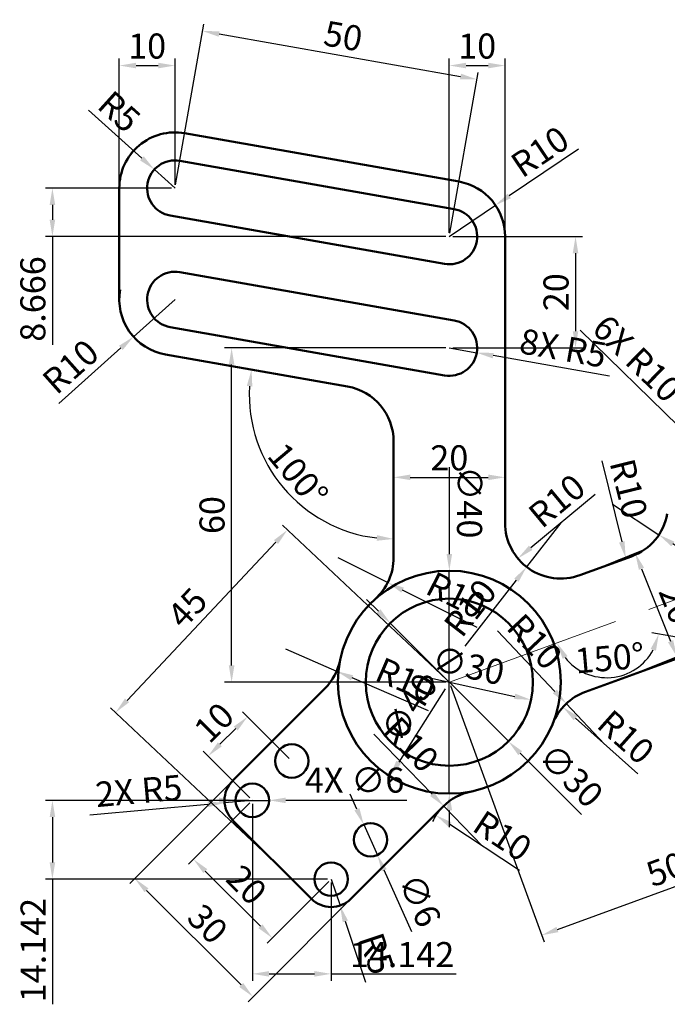
# Model space of a CAD drawing. Units: millimetres. Extents: x 54 to 254, y 16 to 193.
# Tile 1 of 2: x 54 to 170, y 16 to 193. Entities that reach past the tile are written whole.
import ezdxf

# ---------------------------------------------------------------- set-up
doc = ezdxf.new("R2010")
doc.units = ezdxf.units.MM
doc.linetypes.add('CENTER', pattern=[50.8, 31.75, -6.35, 6.35, -6.35])
for name, color, linetype, lineweight in [('M-CNTR', 1, 'CENTER', 18), ('M-DIMS', 2, 'Continuous', 25), ('M-OUTL', 7, 'Continuous', 50)]:
    doc.layers.add(name, color=color, linetype=linetype, lineweight=lineweight)
doc.styles.get("Standard").update_dxf_attribs({"font": 'arial.ttf'})
doc.dimstyles.new('ISO-25', dxfattribs={"dimtxt": 4.5, "dimasz": 3, "dimexe": 1.25, "dimexo": 0.625, "dimtad": 1, "dimdec": 0, "dimtxsty": 'Standard', "dimcen": 2.5, "dimadec": 0, "dimazin": 0, "dimtfac": 1, "dimtdec": 0, "dimtmove": 0, "dimatfit": 3, "dimfxl": 1, "dimarcsym": 0})

# ---------------------------------------------------------------- blocks, each defined once
blk = doc.blocks.new('*D1')
at = {"layer": 'Defpoints', "color": 0, "transparency": 16777216}
for p in [(136.17, 181.85), (81.97, 162.32), (131.21, 153.65)]:
    blk.add_point(p, dxfattribs=at)
at = {"layer": 'M-DIMS', "color": 0, "lineweight": -2, "transparency": 16777216}
for p, q in [((82.08, 162.94), (87.15, 191.75)), ((89.88, 190), (133.22, 182.37)), ((131.32, 154.27), (136.39, 183.08))]:
    blk.add_line(p, q, dxfattribs=at)
at = {"layer": 'M-DIMS', "color": 0, "transparency": 16777216}
for points in [[(89.97, 190.49), (89.8, 189.51), (86.93, 190.52)], [(133.31, 182.87), (133.13, 181.88), (136.17, 181.85)]]:
    blk.add_solid(points, dxfattribs=at)
at = {"layer": 'M-DIMS', "color": 0, "transparency": 16777216, "insert": (112.06, 189.06), "char_height": 4.5, "attachment_point": 5, "rotation": 350.0194}
blk.add_mtext('50', dxfattribs=at)
blk = doc.blocks.new('*D3')
at = {"layer": 'Defpoints', "color": 0, "transparency": 16777216}
for p in [(131.21, 153.65), (131.21, 133.65), (153.86, 133.65)]:
    blk.add_point(p, dxfattribs=at)
at = {"layer": 'M-DIMS', "color": 0, "lineweight": -2, "transparency": 16777216}
for p, q in [((131.84, 153.65), (155.11, 153.65)), ((153.86, 150.65), (153.86, 136.65)), ((131.84, 133.65), (155.11, 133.65))]:
    blk.add_line(p, q, dxfattribs=at)
at = {"layer": 'M-DIMS', "color": 0, "transparency": 16777216}
for points in [[(153.36, 150.65), (154.36, 150.65), (153.86, 153.65)], [(153.36, 136.65), (154.36, 136.65), (153.86, 133.65)]]:
    blk.add_solid(points, dxfattribs=at)
at = {"layer": 'M-DIMS', "color": 0, "transparency": 16777216, "insert": (150.94, 143.65), "char_height": 4.5, "attachment_point": 5, "rotation": 90}
blk.add_mtext('20', dxfattribs=at)
blk = doc.blocks.new('*D4')
at = {"layer": 'Defpoints', "color": 0, "transparency": 16777216}
for p in [(131.21, 73.65), (71.3, 68.2), (100.36, 40.86)]:
    blk.add_point(p, dxfattribs=at)
at = {"layer": 'M-DIMS', "color": 0, "lineweight": -2, "transparency": 16777216}
for p, q in [((130.76, 74.08), (101.24, 101.85)), ((100.09, 98.81), (73.36, 70.38)), ((99.91, 41.29), (70.39, 69.05))]:
    blk.add_line(p, q, dxfattribs=at)
at = {"layer": 'M-DIMS', "color": 0, "transparency": 16777216}
for points in [[(99.73, 99.15), (100.46, 98.46), (102.15, 100.99)], [(72.99, 70.73), (73.72, 70.04), (71.3, 68.2)]]:
    blk.add_solid(points, dxfattribs=at)
at = {"layer": 'M-DIMS', "color": 0, "transparency": 16777216, "insert": (84.6, 86.59), "char_height": 4.5, "attachment_point": 5, "rotation": 46.7521}
blk.add_mtext('45', dxfattribs=at)
blk = doc.blocks.new('*D5')
at = {"layer": 'Defpoints', "color": 0, "transparency": 16777216}
for p in [(94.98, 67.45), (102.93, 59.51), (95.86, 52.44)]:
    blk.add_point(p, dxfattribs=at)
at = {"layer": 'M-DIMS', "color": 0, "lineweight": -2, "transparency": 16777216}
for p, q in [((102.48, 59.95), (94.1, 68.34)), ((90.03, 62.5), (92.86, 65.33)), ((95.41, 52.88), (87.03, 61.27))]:
    blk.add_line(p, q, dxfattribs=at)
at = {"layer": 'M-DIMS', "color": 0, "transparency": 16777216}
for points in [[(92.51, 65.69), (93.22, 64.98), (94.98, 67.45)], [(89.68, 62.86), (90.39, 62.15), (87.91, 60.38)]]:
    blk.add_solid(points, dxfattribs=at)
at = {"layer": 'M-DIMS', "color": 0, "transparency": 16777216, "insert": (89.38, 65.99), "char_height": 4.5, "attachment_point": 5, "rotation": 45}
blk.add_mtext('10', dxfattribs=at)
blk = doc.blocks.new('*D6')
at = {"layer": 'Defpoints', "color": 0, "transparency": 16777216}
for p in [(95.86, 52.44), (85.29, 41.87), (110, 38.3)]:
    blk.add_point(p, dxfattribs=at)
at = {"layer": 'M-DIMS', "color": 0, "lineweight": -2, "transparency": 16777216}
for p, q in [((95.41, 52), (84.4, 40.99)), ((97.31, 29.85), (87.41, 39.75)), ((109.56, 37.86), (98.54, 26.84))]:
    blk.add_line(p, q, dxfattribs=at)
at = {"layer": 'M-DIMS', "color": 0, "transparency": 16777216}
for points in [[(87.76, 40.1), (87.05, 39.4), (85.29, 41.87)], [(97.66, 30.2), (96.95, 29.5), (99.43, 27.73)]]:
    blk.add_solid(points, dxfattribs=at)
at = {"layer": 'M-DIMS', "color": 0, "transparency": 16777216, "insert": (94.42, 36.87), "char_height": 4.5, "attachment_point": 5, "rotation": 315}
blk.add_mtext('20', dxfattribs=at)
blk = doc.blocks.new('*D7')
at = {"layer": 'Defpoints', "color": 0, "transparency": 16777216}
for p in [(95.64, 59.29), (116.85, 38.08), (95.96, 17.19)]:
    blk.add_point(p, dxfattribs=at)
at = {"layer": 'M-DIMS', "color": 0, "lineweight": -2, "transparency": 16777216}
for p, q in [((95.2, 58.85), (73.87, 37.52)), ((116.41, 37.64), (95.08, 16.31)), ((76.87, 36.28), (93.84, 19.31))]:
    blk.add_line(p, q, dxfattribs=at)
at = {"layer": 'M-DIMS', "color": 0, "transparency": 16777216}
for points in [[(77.22, 36.64), (76.52, 35.93), (74.75, 38.41)], [(94.2, 19.67), (93.49, 18.96), (95.96, 17.19)]]:
    blk.add_solid(points, dxfattribs=at)
at = {"layer": 'M-DIMS', "color": 0, "transparency": 16777216, "insert": (87.42, 29.87), "char_height": 4.5, "attachment_point": 5, "rotation": 315}
blk.add_mtext('30', dxfattribs=at)
blk = doc.blocks.new('*D8')
at = {"layer": 'Defpoints', "color": 0, "transparency": 16777216}
for p in [(115.84, 48.11), (118.3, 42.63)]:
    blk.add_point(p, dxfattribs=at)
at = {"layer": 'M-DIMS', "color": 0, "lineweight": -2, "transparency": 16777216}
for p, q in [((114.61, 50.84), (113.39, 53.58)), ((115.84, 48.11), (118.3, 42.63)), ((124.47, 28.86), (119.52, 39.89))]:
    blk.add_line(p, q, dxfattribs=at)
at = {"layer": 'M-DIMS', "color": 0, "transparency": 16777216}
for points in [[(115.07, 51.05), (114.16, 50.64), (115.84, 48.11)], [(119.98, 40.1), (119.07, 39.69), (118.3, 42.63)]]:
    blk.add_solid(points, dxfattribs=at)
at = {"layer": 'M-DIMS', "color": 0, "transparency": 16777216, "insert": (125.39, 34.26), "char_height": 4.5, "attachment_point": 5, "rotation": 294.1535}
blk.add_mtext('∅6', dxfattribs=at)
blk = doc.blocks.new('*D9')
at = {"layer": 'Defpoints', "color": 0, "transparency": 16777216}
for p in [(110, 38.3), (111.59, 33.56)]:
    blk.add_point(p, dxfattribs=at)
at = {"layer": 'M-DIMS', "color": 0, "lineweight": -2, "transparency": 16777216}
for p, q in [((110, 38.3), (111.59, 33.56)), ((116.22, 19.78), (112.55, 30.72))]:
    blk.add_line(p, q, dxfattribs=at)
at = {"layer": 'M-DIMS', "color": 0, "transparency": 16777216}
blk.add_solid([(113.02, 30.87), (112.07, 30.56), (111.59, 33.56)], dxfattribs=at)
at = {"layer": 'M-DIMS', "color": 0, "transparency": 16777216, "insert": (117.63, 24.75), "char_height": 4.5, "attachment_point": 5, "rotation": 288.5828}
blk.add_mtext('R5', dxfattribs=at)
blk = doc.blocks.new('*D10')
at = {"layer": 'Defpoints', "color": 0, "transparency": 16777216}
for p in [(128.82, 49.76), (137.16, 44.25)]:
    blk.add_point(p, dxfattribs=at)
at = {"layer": 'M-DIMS', "color": 0, "lineweight": -2, "transparency": 16777216}
blk.add_line((143.83, 39.85), (131.32, 48.11), dxfattribs=at)
blk.add_arc((137.16, 44.25), 10, 138.581, 153.7241, dxfattribs=at)
at = {"layer": 'M-DIMS', "color": 0, "transparency": 16777216}
blk.add_solid([(131.6, 48.52), (131.05, 47.69), (128.82, 49.76)], dxfattribs=at)
at = {"layer": 'M-DIMS', "color": 0, "transparency": 16777216, "insert": (140.44, 45.59), "char_height": 4.5, "attachment_point": 5, "rotation": 326.5622}
blk.add_mtext('R10', dxfattribs=at)
blk = doc.blocks.new('*D11')
at = {"layer": 'Defpoints', "color": 0, "transparency": 16777216}
for p in [(116.55, 76.83), (145.87, 70.48)]:
    blk.add_point(p, dxfattribs=at)
at = {"layer": 'M-DIMS', "color": 0, "lineweight": -2, "transparency": 16777216}
blk.add_line((127.71, 74.41), (142.94, 71.11), dxfattribs=at)
at = {"layer": 'M-DIMS', "color": 0, "transparency": 16777216}
blk.add_solid([(143.04, 71.6), (142.83, 70.63), (145.87, 70.48)], dxfattribs=at)
at = {"layer": 'M-DIMS', "color": 0, "transparency": 16777216, "insert": (134.51, 76.06), "char_height": 4.5, "attachment_point": 5, "rotation": 347.7817}
blk.add_mtext('∅30', dxfattribs=at)
blk = doc.blocks.new('*D12')
at = {"layer": 'Defpoints', "color": 0, "transparency": 16777216}
for p in [(141.9, 90.56), (120.52, 56.75)]:
    blk.add_point(p, dxfattribs=at)
at = {"layer": 'M-DIMS', "color": 0, "lineweight": -2, "transparency": 16777216}
blk.add_line((130.45, 72.45), (122.12, 59.29), dxfattribs=at)
at = {"layer": 'M-DIMS', "color": 0, "transparency": 16777216}
blk.add_solid([(121.7, 59.55), (122.55, 59.02), (120.52, 56.75)], dxfattribs=at)
at = {"layer": 'M-DIMS', "color": 0, "transparency": 16777216, "insert": (124.51, 68.77), "char_height": 4.5, "attachment_point": 5, "rotation": 57.6851}
blk.add_mtext('∅40', dxfattribs=at)
blk = doc.blocks.new('*D13')
at = {"layer": 'Defpoints', "color": 0, "transparency": 16777216}
for p in [(139.49, 159.26), (131.21, 153.65)]:
    blk.add_point(p, dxfattribs=at)
at = {"layer": 'M-DIMS', "color": 0, "lineweight": -2, "transparency": 16777216}
for p, q in [((154.4, 169.33), (141.98, 160.94)), ((131.21, 153.65), (139.49, 159.26))]:
    blk.add_line(p, q, dxfattribs=at)
at = {"layer": 'M-DIMS', "color": 0, "transparency": 16777216}
blk.add_solid([(141.7, 161.35), (142.26, 160.52), (139.49, 159.26)], dxfattribs=at)
at = {"layer": 'M-DIMS', "color": 0, "transparency": 16777216, "insert": (147.79, 168.39), "char_height": 4.5, "attachment_point": 5, "rotation": 34.0663}
blk.add_mtext('R10', dxfattribs=at)
blk = doc.blocks.new('*D14')
at = {"layer": 'Defpoints', "color": 0, "transparency": 16777216}
for p in [(78.26, 165.67), (81.97, 162.32)]:
    blk.add_point(p, dxfattribs=at)
at = {"layer": 'M-DIMS', "color": 0, "lineweight": -2, "transparency": 16777216}
for p, q in [((66.45, 176.32), (76.03, 167.68)), ((81.97, 162.32), (78.26, 165.67))]:
    blk.add_line(p, q, dxfattribs=at)
at = {"layer": 'M-DIMS', "color": 0, "transparency": 16777216}
blk.add_solid([(76.36, 168.05), (75.69, 167.31), (78.26, 165.67)], dxfattribs=at)
at = {"layer": 'M-DIMS', "color": 0, "transparency": 16777216, "insert": (71.58, 175.63), "char_height": 4.5, "attachment_point": 5, "rotation": 317.9238}
blk.add_mtext('R5', dxfattribs=at)
blk = doc.blocks.new('*D15')
at = {"layer": 'Defpoints', "color": 0, "transparency": 16777216}
for p in [(81.97, 142.32), (74.51, 135.66)]:
    blk.add_point(p, dxfattribs=at)
at = {"layer": 'M-DIMS', "color": 0, "lineweight": -2, "transparency": 16777216}
for p, q in [((81.97, 142.32), (74.51, 135.66)), ((61.09, 123.68), (72.27, 133.66))]:
    blk.add_line(p, q, dxfattribs=at)
at = {"layer": 'M-DIMS', "color": 0, "transparency": 16777216}
blk.add_solid([(71.93, 134.04), (72.6, 133.29), (74.51, 135.66)], dxfattribs=at)
at = {"layer": 'M-DIMS', "color": 0, "transparency": 16777216, "insert": (63.61, 129.86), "char_height": 4.5, "attachment_point": 5, "rotation": 41.7451}
blk.add_mtext('R10', dxfattribs=at)
blk = doc.blocks.new('*D16')
at = {"layer": 'Defpoints', "color": 0, "transparency": 16777216}
for p in [(80.23, 132.47), (112.94, 126.71), (121.21, 116.87), (97.43, 115), (121.21, 96.01)]:
    blk.add_point(p, dxfattribs=at)
at = {"layer": 'M-DIMS', "color": 0, "lineweight": -2, "transparency": 16777216}
blk.add_arc((121.21, 125.26), 25.9, 176.6604, 263.359, dxfattribs=at)
at = {"layer": 'M-DIMS', "color": 0, "transparency": 16777216}
for points in [[(94.86, 126.83), (95.85, 126.71), (95.71, 129.75)], [(118.24, 100.04), (118.19, 99.04), (121.21, 99.36)]]:
    blk.add_solid(points, dxfattribs=at)
at = {"layer": 'M-DIMS', "color": 0, "transparency": 16777216, "insert": (103.61, 110.49), "char_height": 4.5, "attachment_point": 5, "rotation": 310.0097}
blk.add_mtext('100°', dxfattribs=at)
blk = doc.blocks.new('*D17')
at = {"layer": 'Defpoints', "color": 0, "transparency": 16777216}
for p in [(92.13, 133.65), (131.21, 133.65), (131.21, 73.65)]:
    blk.add_point(p, dxfattribs=at)
at = {"layer": 'M-DIMS', "color": 0, "lineweight": -2, "transparency": 16777216}
for p, q in [((130.59, 133.65), (90.88, 133.65)), ((92.13, 76.65), (92.13, 130.65)), ((130.59, 73.65), (90.88, 73.65))]:
    blk.add_line(p, q, dxfattribs=at)
at = {"layer": 'M-DIMS', "color": 0, "transparency": 16777216}
for points in [[(91.63, 130.65), (92.63, 130.65), (92.13, 133.65)], [(91.63, 76.65), (92.63, 76.65), (92.13, 73.65)]]:
    blk.add_solid(points, dxfattribs=at)
at = {"layer": 'M-DIMS', "color": 0, "transparency": 16777216, "insert": (89.2, 103.65), "char_height": 4.5, "attachment_point": 5, "rotation": 90}
blk.add_mtext('60', dxfattribs=at)
blk = doc.blocks.new('*D18')
at = {"layer": 'Defpoints', "color": 0, "transparency": 16777216}
for p in [(151.21, 102.24), (143.51, 95.86)]:
    blk.add_point(p, dxfattribs=at)
at = {"layer": 'M-DIMS', "color": 0, "lineweight": -2, "transparency": 16777216}
blk.add_line((157.36, 107.34), (145.82, 97.78), dxfattribs=at)
at = {"layer": 'M-DIMS', "color": 0, "transparency": 16777216}
blk.add_solid([(145.5, 98.16), (146.14, 97.39), (143.51, 95.86)], dxfattribs=at)
at = {"layer": 'M-DIMS', "color": 0, "transparency": 16777216, "insert": (150.88, 105.76), "char_height": 4.5, "attachment_point": 5, "rotation": 39.6266}
blk.add_mtext('R10', dxfattribs=at)
blk = doc.blocks.new('*D19')
at = {"layer": 'Defpoints', "color": 0, "transparency": 16777216}
for p in [(160.49, 105.63), (162.88, 95.92)]:
    blk.add_point(p, dxfattribs=at)
at = {"layer": 'M-DIMS', "color": 0, "lineweight": -2, "transparency": 16777216}
blk.add_line((158.58, 113.38), (162.16, 98.83), dxfattribs=at)
blk.add_arc((160.49, 105.63), 10, 276.6667, 286.4669, dxfattribs=at)
at = {"layer": 'M-DIMS', "color": 0, "transparency": 16777216}
blk.add_solid([(162.65, 98.95), (161.68, 98.71), (162.88, 95.92)], dxfattribs=at)
at = {"layer": 'M-DIMS', "color": 0, "transparency": 16777216, "insert": (162.85, 108.26), "char_height": 4.5, "attachment_point": 5, "rotation": 283.8287}
blk.add_mtext('R10', dxfattribs=at)
blk = doc.blocks.new('*D20')
at = {"layer": 'Defpoints', "color": 0, "transparency": 16777216}
for p in [(155.74, 93.25), (172.04, 78.24), (163.21, 74.69)]:
    blk.add_point(p, dxfattribs=at)
at = {"layer": 'M-DIMS', "color": 0, "lineweight": -2, "transparency": 16777216}
for p, q in [((156.32, 93.48), (165.74, 97.27)), ((165.7, 94.02), (170.92, 81.02)), ((163.79, 74.92), (173.2, 78.7))]:
    blk.add_line(p, q, dxfattribs=at)
at = {"layer": 'M-DIMS', "color": 0, "transparency": 16777216}
for points in [[(166.16, 94.21), (165.23, 93.83), (164.58, 96.8)], [(171.39, 81.21), (170.46, 80.83), (172.04, 78.24)]]:
    blk.add_solid(points, dxfattribs=at)
at = {"layer": 'M-DIMS', "color": 0, "transparency": 16777216, "insert": (171.5, 87.42), "char_height": 4.5, "attachment_point": 5, "rotation": 291.9033}
blk.add_mtext('20', dxfattribs=at)
blk = doc.blocks.new('*D21')
at = {"layer": 'Defpoints', "color": 0, "transparency": 16777216}
for p in [(151.61, 69.19), (159.07, 62.53)]:
    blk.add_point(p, dxfattribs=at)
at = {"layer": 'M-DIMS', "color": 0, "lineweight": -2, "transparency": 16777216}
blk.add_line((165.03, 57.21), (153.85, 67.19), dxfattribs=at)
at = {"layer": 'M-DIMS', "color": 0, "transparency": 16777216}
blk.add_solid([(154.19, 67.57), (153.52, 66.82), (151.61, 69.19)], dxfattribs=at)
at = {"layer": 'M-DIMS', "color": 0, "transparency": 16777216, "insert": (162.51, 63.38), "char_height": 4.5, "attachment_point": 5, "rotation": 318.2256}
blk.add_mtext('R10', dxfattribs=at)
blk = doc.blocks.new('*D22')
at = {"layer": 'Defpoints', "color": 0, "transparency": 16777216}
for p in [(121.21, 110.07), (141.21, 110.42), (141.21, 110.07)]:
    blk.add_point(p, dxfattribs=at)
at = {"layer": 'M-DIMS', "color": 0, "lineweight": -2, "transparency": 16777216}
for p, q in [((121.21, 110.69), (121.21, 111.67)), ((141.21, 110.69), (141.21, 111.67)), ((124.21, 110.42), (138.21, 110.42))]:
    blk.add_line(p, q, dxfattribs=at)
at = {"layer": 'M-DIMS', "color": 0, "transparency": 16777216}
for points in [[(124.21, 110.92), (124.21, 109.92), (121.21, 110.42)], [(138.21, 110.92), (138.21, 109.92), (141.21, 110.42)]]:
    blk.add_solid(points, dxfattribs=at)
at = {"layer": 'M-DIMS', "color": 0, "transparency": 16777216, "insert": (131.21, 113.34), "char_height": 4.5, "attachment_point": 5}
blk.add_mtext('20', dxfattribs=at)
blk = doc.blocks.new('*D24')
at = {"layer": 'Defpoints', "color": 0, "transparency": 16777216}
for p in [(178.18, 90.79), (131.21, 73.65), (194.76, 45.37)]:
    blk.add_point(p, dxfattribs=at)
at = {"layer": 'M-DIMS', "color": 0, "lineweight": -2, "transparency": 16777216}
for p, q in [((178.4, 90.21), (195.19, 44.19)), ((131.42, 73.07), (148.22, 27.05)), ((150.61, 29.26), (191.94, 44.34))]:
    blk.add_line(p, q, dxfattribs=at)
at = {"layer": 'M-DIMS', "color": 0, "transparency": 16777216}
for points in [[(191.77, 44.81), (192.11, 43.87), (194.76, 45.37)], [(150.43, 29.73), (150.78, 28.79), (147.79, 28.23)]]:
    blk.add_solid(points, dxfattribs=at)
at = {"layer": 'M-DIMS', "color": 0, "transparency": 16777216, "insert": (170.27, 39.54), "char_height": 4.5, "attachment_point": 5, "rotation": 20.0485}
blk.add_mtext('50', dxfattribs=at)
blk = doc.blocks.new('*D27')
at = {"layer": 'Defpoints', "color": 0, "transparency": 16777216}
for p in [(178.18, 90.79), (181.73, 80.01), (156.21, 75.03), (131.21, 73.65), (225.67, 72.21)]:
    blk.add_point(p, dxfattribs=at)
at = {"layer": 'M-DIMS', "color": 0, "lineweight": -2, "transparency": 16777216}
blk.add_line((181.12, 80.12), (167.58, 82.52), dxfattribs=at)
blk.add_arc((159.45, 83.96), 9.5, 218.2164, 331.7726, dxfattribs=at)
at = {"layer": 'M-DIMS', "color": 0, "transparency": 16777216}
for points in [[(167.35, 79.63), (168.3, 79.3), (168.81, 82.3)], [(151.55, 77.84), (152.43, 78.33), (150.53, 80.7)]]:
    blk.add_solid(points, dxfattribs=at)
at = {"layer": 'M-DIMS', "color": 0, "transparency": 16777216, "insert": (160.03, 77.41), "char_height": 4.5, "attachment_point": 5, "rotation": 4.9945}
blk.add_mtext('150°', dxfattribs=at)
blk = doc.blocks.new('*D29')
at = {"layer": 'Defpoints', "color": 0, "transparency": 16777216}
for p in [(81.97, 184.33), (71.97, 162.34), (81.97, 162.32)]:
    blk.add_point(p, dxfattribs=at)
at = {"layer": 'M-DIMS', "color": 0, "lineweight": -2, "transparency": 16777216}
for p, q in [((71.97, 162.96), (71.97, 185.58)), ((81.97, 162.94), (81.97, 185.58)), ((74.97, 184.33), (78.97, 184.33))]:
    blk.add_line(p, q, dxfattribs=at)
at = {"layer": 'M-DIMS', "color": 0, "transparency": 16777216}
for points in [[(74.97, 184.83), (74.97, 183.83), (71.97, 184.33)], [(78.97, 184.83), (78.97, 183.83), (81.97, 184.33)]]:
    blk.add_solid(points, dxfattribs=at)
at = {"layer": 'M-DIMS', "color": 0, "transparency": 16777216, "insert": (76.97, 187.25), "char_height": 4.5, "attachment_point": 5}
blk.add_mtext('10', dxfattribs=at)
blk = doc.blocks.new('*D30')
at = {"layer": 'Defpoints', "color": 0, "transparency": 16777216}
for p in [(141.21, 184.33), (131.21, 153.65), (141.21, 153.65)]:
    blk.add_point(p, dxfattribs=at)
at = {"layer": 'M-DIMS', "color": 0, "lineweight": -2, "transparency": 16777216}
for p, q in [((131.21, 154.28), (131.21, 185.58)), ((141.21, 154.28), (141.21, 185.58)), ((134.21, 184.33), (138.21, 184.33))]:
    blk.add_line(p, q, dxfattribs=at)
at = {"layer": 'M-DIMS', "color": 0, "transparency": 16777216}
for points in [[(134.21, 184.83), (134.21, 183.83), (131.21, 184.33)], [(138.21, 184.83), (138.21, 183.83), (141.21, 184.33)]]:
    blk.add_solid(points, dxfattribs=at)
at = {"layer": 'M-DIMS', "color": 0, "transparency": 16777216, "insert": (136.21, 187.25), "char_height": 4.5, "attachment_point": 5}
blk.add_mtext('10', dxfattribs=at)
blk = doc.blocks.new('*D31')
at = {"layer": 'Defpoints', "color": 0, "transparency": 16777216}
for p in [(81.97, 162.32), (59.97, 153.65), (131.21, 153.65)]:
    blk.add_point(p, dxfattribs=at)
at = {"layer": 'M-DIMS', "color": 0, "lineweight": -2, "transparency": 16777216}
for p, q in [((81.34, 162.32), (58.72, 162.32)), ((59.97, 159.32), (59.97, 156.65)), ((130.59, 153.65), (58.72, 153.65)), ((59.97, 153.65), (59.97, 134.22))]:
    blk.add_line(p, q, dxfattribs=at)
at = {"layer": 'M-DIMS', "color": 0, "transparency": 16777216}
for points in [[(59.47, 159.32), (60.47, 159.32), (59.97, 162.32)], [(59.47, 156.65), (60.47, 156.65), (59.97, 153.65)]]:
    blk.add_solid(points, dxfattribs=at)
at = {"layer": 'M-DIMS', "color": 0, "transparency": 16777216, "insert": (57.04, 142.43), "char_height": 4.5, "attachment_point": 5, "rotation": 90}
blk.add_mtext('8.666', dxfattribs=at)
blk = doc.blocks.new('*D33')
at = {"layer": 'Defpoints', "color": 0, "transparency": 16777216}
for p in [(95.86, 52.44), (59.97, 38.3), (110, 38.3)]:
    blk.add_point(p, dxfattribs=at)
at = {"layer": 'M-DIMS', "color": 0, "lineweight": -2, "transparency": 16777216}
for p, q in [((95.23, 52.44), (58.72, 52.44)), ((59.97, 49.44), (59.97, 41.3)), ((109.37, 38.3), (58.72, 38.3)), ((59.97, 38.3), (59.97, 15.84))]:
    blk.add_line(p, q, dxfattribs=at)
at = {"layer": 'M-DIMS', "color": 0, "transparency": 16777216}
for points in [[(59.47, 49.44), (60.47, 49.44), (59.97, 52.44)], [(59.47, 41.3), (60.47, 41.3), (59.97, 38.3)]]:
    blk.add_solid(points, dxfattribs=at)
at = {"layer": 'M-DIMS', "color": 0, "transparency": 16777216, "insert": (57.08, 25.57), "char_height": 4.5, "attachment_point": 5, "rotation": 90}
blk.add_mtext('14.142', dxfattribs=at)
blk = doc.blocks.new('*D34')
at = {"layer": 'Defpoints', "color": 0, "transparency": 16777216}
for p in [(95.86, 52.44), (110, 38.3), (110, 21.3)]:
    blk.add_point(p, dxfattribs=at)
at = {"layer": 'M-DIMS', "color": 0, "lineweight": -2, "transparency": 16777216}
for p, q in [((95.86, 51.82), (95.86, 20.05)), ((110, 37.67), (110, 20.05)), ((98.86, 21.3), (107, 21.3)), ((110, 21.3), (132.46, 21.3))]:
    blk.add_line(p, q, dxfattribs=at)
at = {"layer": 'M-DIMS', "color": 0, "transparency": 16777216}
for points in [[(98.86, 21.8), (98.86, 20.8), (95.86, 21.3)], [(107, 21.8), (107, 20.8), (110, 21.3)]]:
    blk.add_solid(points, dxfattribs=at)
at = {"layer": 'M-DIMS', "color": 0, "transparency": 16777216, "insert": (122.73, 24.18), "char_height": 4.5, "attachment_point": 5}
blk.add_mtext('14.142', dxfattribs=at)
blk = doc.blocks.new('*D35')
at = {"layer": 'Defpoints', "color": 0, "transparency": 16777216}
for p in [(131.21, 93.65), (131.21, 53.65)]:
    blk.add_point(p, dxfattribs=at)
at = {"layer": 'M-DIMS', "color": 0, "lineweight": -2, "transparency": 16777216}
for p, q in [((131.21, 112.23), (131.21, 96.65)), ((131.21, 53.65), (131.21, 93.65)), ((131.21, 50.65), (131.21, 47.65))]:
    blk.add_line(p, q, dxfattribs=at)
at = {"layer": 'M-DIMS', "color": 0, "transparency": 16777216}
for points in [[(131.71, 96.65), (130.71, 96.65), (131.21, 93.65)], [(131.71, 50.65), (130.71, 50.65), (131.21, 53.65)]]:
    blk.add_solid(points, dxfattribs=at)
at = {"layer": 'M-DIMS', "color": 0, "transparency": 16777216, "insert": (134.26, 105.94), "char_height": 4.5, "attachment_point": 5, "rotation": 270.002}
blk.add_mtext('∅40', dxfattribs=at)
blk = doc.blocks.new('*D36')
at = {"layer": 'Defpoints', "color": 0, "transparency": 16777216}
for p in [(120.61, 84.27), (141.81, 63.04)]:
    blk.add_point(p, dxfattribs=at)
at = {"layer": 'M-DIMS', "color": 0, "lineweight": -2, "transparency": 16777216}
for p, q in [((118.49, 86.39), (116.37, 88.51)), ((120.61, 84.27), (141.81, 63.04)), ((154.94, 49.9), (143.93, 60.92))]:
    blk.add_line(p, q, dxfattribs=at)
at = {"layer": 'M-DIMS', "color": 0, "transparency": 16777216}
for points in [[(118.85, 86.74), (118.14, 86.04), (120.61, 84.27)], [(144.28, 61.27), (143.58, 60.56), (141.81, 63.04)]]:
    blk.add_solid(points, dxfattribs=at)
at = {"layer": 'M-DIMS', "color": 0, "transparency": 16777216, "insert": (152.65, 56.5), "char_height": 4.5, "attachment_point": 5, "rotation": 314.9609}
blk.add_mtext('∅30', dxfattribs=at)
blk = doc.blocks.new('*D37')
at = {"layer": 'Defpoints', "color": 0, "transparency": 16777216}
for p in [(92.86, 52.44), (98.86, 52.44)]:
    blk.add_point(p, dxfattribs=at)
at = {"layer": 'M-DIMS', "color": 0, "lineweight": -2, "transparency": 16777216}
for p, q in [((89.86, 52.44), (86.86, 52.44)), ((92.86, 52.44), (98.86, 52.44)), ((123.56, 52.44), (101.86, 52.44))]:
    blk.add_line(p, q, dxfattribs=at)
at = {"layer": 'M-DIMS', "color": 0, "transparency": 16777216}
for points in [[(89.86, 52.94), (89.86, 51.94), (92.86, 52.44)], [(101.86, 52.94), (101.86, 51.94), (98.86, 52.44)]]:
    blk.add_solid(points, dxfattribs=at)
at = {"layer": 'M-DIMS', "color": 0, "transparency": 16777216, "insert": (114.21, 55.49), "char_height": 4.5, "attachment_point": 5, "rotation": 0.0081}
blk.add_mtext('4X ∅6', dxfattribs=at)
blk = doc.blocks.new('*D38')
at = {"layer": 'Defpoints', "color": 0, "transparency": 16777216}
for p in [(131.21, 133.65), (136.13, 132.79)]:
    blk.add_point(p, dxfattribs=at)
at = {"layer": 'M-DIMS', "color": 0, "lineweight": -2, "transparency": 16777216}
for p, q in [((131.21, 133.65), (136.13, 132.79)), ((159.98, 128.59), (139.09, 132.27))]:
    blk.add_line(p, q, dxfattribs=at)
at = {"layer": 'M-DIMS', "color": 0, "transparency": 16777216}
blk.add_solid([(139.18, 132.76), (139, 131.77), (136.13, 132.79)], dxfattribs=at)
at = {"layer": 'M-DIMS', "color": 0, "transparency": 16777216, "insert": (151.52, 133.05), "char_height": 4.5, "attachment_point": 5, "rotation": 350.017}
blk.add_mtext('8X R5', dxfattribs=at)
blk = doc.blocks.new('*D39')
at = {"layer": 'Defpoints', "color": 0, "transparency": 16777216}
for p in [(90.88, 52), (95.86, 52.44)]:
    blk.add_point(p, dxfattribs=at)
at = {"layer": 'M-DIMS', "color": 0, "lineweight": -2, "transparency": 16777216}
for p, q in [((66.68, 49.85), (87.89, 51.73)), ((95.86, 52.44), (90.88, 52))]:
    blk.add_line(p, q, dxfattribs=at)
at = {"layer": 'M-DIMS', "color": 0, "transparency": 16777216}
blk.add_solid([(87.84, 52.23), (87.93, 51.23), (90.88, 52)], dxfattribs=at)
at = {"layer": 'M-DIMS', "color": 0, "transparency": 16777216, "insert": (75.53, 53.57), "char_height": 4.5, "attachment_point": 5, "rotation": 5.0808}
blk.add_mtext('2X R5', dxfattribs=at)
blk = doc.blocks.new('*D40')
at = {"layer": 'Defpoints', "color": 0, "transparency": 16777216}
for p in [(151.21, 102.24), (145.08, 94.34)]:
    blk.add_point(p, dxfattribs=at)
at = {"layer": 'M-DIMS', "color": 0, "lineweight": -2, "transparency": 16777216}
for p, q in [((151.21, 102.24), (145.08, 94.34)), ((134.06, 80.12), (143.25, 91.97))]:
    blk.add_line(p, q, dxfattribs=at)
at = {"layer": 'M-DIMS', "color": 0, "transparency": 16777216}
blk.add_solid([(142.85, 92.27), (143.64, 91.66), (145.08, 94.34)], dxfattribs=at)
at = {"layer": 'M-DIMS', "color": 0, "transparency": 16777216, "insert": (135.42, 86.65), "char_height": 4.5, "attachment_point": 5, "rotation": 52.2124}
blk.add_mtext('R10', dxfattribs=at)
blk = doc.blocks.new('*D41')
at = {"layer": 'Defpoints', "color": 0, "transparency": 16777216}
for p in [(160.49, 105.63), (168.83, 100.11)]:
    blk.add_point(p, dxfattribs=at)
at = {"layer": 'M-DIMS', "color": 0, "lineweight": -2, "transparency": 16777216}
for p, q in [((160.49, 105.63), (168.83, 100.11)), ((183.83, 90.19), (171.33, 98.46))]:
    blk.add_line(p, q, dxfattribs=at)
at = {"layer": 'M-DIMS', "color": 0, "transparency": 16777216}
blk.add_solid([(171.61, 98.88), (171.06, 98.04), (168.83, 100.11)], dxfattribs=at)
at = {"layer": 'M-DIMS', "color": 0, "transparency": 16777216, "insert": (180.45, 95.94), "char_height": 4.5, "attachment_point": 5, "rotation": 326.5309}
blk.add_mtext('R10', dxfattribs=at)
blk = doc.blocks.new('*D42')
at = {"layer": 'Defpoints', "color": 0, "transparency": 16777216}
for p in [(152.21, 69.81), (159.07, 62.53)]:
    blk.add_point(p, dxfattribs=at)
at = {"layer": 'M-DIMS', "color": 0, "lineweight": -2, "transparency": 16777216}
for p, q in [((139.87, 82.89), (150.15, 71.99)), ((159.07, 62.53), (152.21, 69.81))]:
    blk.add_line(p, q, dxfattribs=at)
at = {"layer": 'M-DIMS', "color": 0, "transparency": 16777216}
blk.add_solid([(150.52, 72.33), (149.79, 71.65), (152.21, 69.81)], dxfattribs=at)
at = {"layer": 'M-DIMS', "color": 0, "transparency": 16777216, "insert": (146.11, 80.54), "char_height": 4.5, "attachment_point": 5, "rotation": 313.3232}
blk.add_mtext('R10', dxfattribs=at)
blk = doc.blocks.new('*D43')
at = {"layer": 'Defpoints', "color": 0, "transparency": 16777216}
for p in [(130.2, 51.43), (137.16, 44.25)]:
    blk.add_point(p, dxfattribs=at)
at = {"layer": 'M-DIMS', "color": 0, "lineweight": -2, "transparency": 16777216}
for p, q in [((117.67, 64.33), (128.11, 53.58)), ((137.16, 44.25), (130.2, 51.43))]:
    blk.add_line(p, q, dxfattribs=at)
at = {"layer": 'M-DIMS', "color": 0, "transparency": 16777216}
blk.add_solid([(128.47, 53.93), (127.75, 53.23), (130.2, 51.43)], dxfattribs=at)
at = {"layer": 'M-DIMS', "color": 0, "transparency": 16777216, "insert": (123.94, 62.07), "char_height": 4.5, "attachment_point": 5, "rotation": 314.141}
blk.add_mtext('R10', dxfattribs=at)
blk = doc.blocks.new('*D44')
at = {"layer": 'Defpoints', "color": 0, "transparency": 16777216}
for p in [(101.81, 79.61), (110.98, 75.63)]:
    blk.add_point(p, dxfattribs=at)
at = {"layer": 'M-DIMS', "color": 0, "lineweight": -2, "transparency": 16777216}
for p, q in [((101.81, 79.61), (110.98, 75.63)), ((127.49, 68.49), (113.74, 74.44))]:
    blk.add_line(p, q, dxfattribs=at)
at = {"layer": 'M-DIMS', "color": 0, "transparency": 16777216}
blk.add_solid([(113.94, 74.9), (113.54, 73.98), (110.98, 75.63)], dxfattribs=at)
at = {"layer": 'M-DIMS', "color": 0, "transparency": 16777216, "insert": (123.15, 73.55), "char_height": 4.5, "attachment_point": 5, "rotation": 336.5982}
blk.add_mtext('R10', dxfattribs=at)
blk = doc.blocks.new('*D45')
at = {"layer": 'Defpoints', "color": 0, "transparency": 16777216}
for p in [(111.21, 96.01), (120.15, 91.53)]:
    blk.add_point(p, dxfattribs=at)
at = {"layer": 'M-DIMS', "color": 0, "lineweight": -2, "transparency": 16777216}
for p, q in [((111.21, 96.01), (120.15, 91.53)), ((136.22, 83.45), (122.83, 90.18))]:
    blk.add_line(p, q, dxfattribs=at)
at = {"layer": 'M-DIMS', "color": 0, "transparency": 16777216}
blk.add_solid([(123.05, 90.63), (122.6, 89.73), (120.15, 91.53)], dxfattribs=at)
at = {"layer": 'M-DIMS', "color": 0, "transparency": 16777216, "insert": (132.18, 88.76), "char_height": 4.5, "attachment_point": 5, "rotation": 333.334}
blk.add_mtext('R10', dxfattribs=at)
blk = doc.blocks.new('*D46')
at = {"layer": 'Defpoints', "color": 0, "transparency": 16777216}
for p in [(174.51, 117.48), (181.65, 110.49)]:
    blk.add_point(p, dxfattribs=at)
at = {"layer": 'M-DIMS', "color": 0, "lineweight": -2, "transparency": 16777216}
for p, q in [((154.72, 136.84), (172.36, 119.58)), ((181.65, 110.49), (174.51, 117.48))]:
    blk.add_line(p, q, dxfattribs=at)
at = {"layer": 'M-DIMS', "color": 0, "transparency": 16777216}
blk.add_solid([(172.71, 119.94), (172.01, 119.22), (174.51, 117.48)], dxfattribs=at)
at = {"layer": 'M-DIMS', "color": 0, "transparency": 16777216, "insert": (164.51, 131.35), "char_height": 4.5, "attachment_point": 5, "rotation": 315.6289}
blk.add_mtext('6X R10', dxfattribs=at)

msp = doc.modelspace()

# ---------------------------------------------------------------- linework, layer by layer
at = {"layer": 'M-CNTR'}
msp.add_line((131.2107, 73.6538), (178.1808, 90.7945), dxfattribs=at)
at = {"layer": 'M-OUTL'}
for p, q in [((83.7039, 172.1848), (132.9472, 163.5019)), ((71.9674, 142.3195), (71.9674, 162.3367)), ((141.2107, 153.6538), (141.2107, 133.6538)), ((141.2107, 102.2422), (141.2107, 133.6538)), ((80.2342, 132.4708), (112.9438, 126.7147)), ((121.2107, 96.0145), (121.2107, 116.866)), ((154.6388, 92.8481), (163.9158, 96.2335)), ((155.6445, 71.9251), (176.5568, 79.5563)), ((108.8781, 72.5343), (92.3198, 55.9761)), ((130.0913, 51.3211), (113.533, 34.7629)), ((92.3198, 48.905), (106.462, 34.7629))]:
    msp.add_line(p, q, dxfattribs=at)
for points in [[(130.3441, 148.7294, 1), (132.0773, 158.5781), (82.8339, 167.2438, 1), (81.1008, 157.3952)], [(130.3441, 128.7294, 1), (132.0773, 138.5781), (82.8339, 147.2438, 1), (81.1008, 137.3952)]]:
    msp.add_lwpolyline(points, format="xyb", close=True, dxfattribs=at)
for centre, radius in [((131.2107, 73.6538), 20), ((131.2107, 73.6538), 15), ((102.9264, 59.5116), 3), ((95.8554, 52.4406), 3), ((117.0686, 45.3695), 3), ((109.9975, 38.2984), 3)]:
    msp.add_circle(centre, radius, dxfattribs=at)
for centre, radius, start, end in [((81.9674, 162.3367), 10, 80, 180), ((131.2107, 153.6538), 10, 0, 80), ((81.9674, 142.3195), 10, 169.902938, 260.019412), ((111.2107, 116.866), 10, 0, 80.019412), ((160.4878, 105.6275), 10, 290.047893, 350), ((151.2107, 102.2422), 10, 180, 290.047893), ((111.2107, 96.0145), 10, 311.810315, 360), ((101.807, 79.6054), 10, 315, 348.55731), ((159.0726, 62.531), 10, 110.047893, 158.237578), ((95.8554, 52.4406), 5, 135, 225), ((137.1623, 44.2501), 10, 101.44269, 135), ((109.9975, 38.2984), 5, 225, 315)]:
    msp.add_arc(centre, radius, start, end, dxfattribs=at)

# ---------------------------------------------------------------- dimensions: what is measured, and where the dimension line sits
at = {"layer": 'M-DIMS'}
for p1, p2, distance, picture, middle in [((81.9674, 162.3195), (131.2107, 153.6538), 28.6324, '*D1', (112.058, 189.0641)), ((131.2107, 153.6538), (131.2107, 133.6538), 22.6536, '*D3', (150.9417, 143.6538)), ((131.2107, 73.6538), (100.3643, 40.8606), -39.8984, '*D4', (84.6035, 86.59)), ((131.2107, 73.6538), (178.1808, 90.7945), -48.356, '*D24', (170.271, 39.5439)), ((95.8554, 52.4406), (102.9264, 59.5116), 11.2331, '*D5', (89.3813, 65.9857)), ((95.6381, 59.2944), (116.8513, 38.0812), -29.5407, '*D7', (87.4239, 29.867)), ((109.9975, 38.2984), (95.8554, 52.4406), 14.9479, '*D6', (94.4232, 36.8663))]:
    dim = msp.add_aligned_dim(p1=p1, p2=p2, distance=distance, dimstyle='ISO-25', override={"dimclrd": 0, "dimclre": 0, "dimclrt": 0}, dxfattribs=at)
    dim.commit()
    dim.dimension.update_dxf_attribs({"geometry": picture, "text_midpoint": middle})
for base, p1, p2, override, picture, middle in [((81.9674, 184.3267), (71.9674, 162.3367), (81.9674, 162.3195), {"dimdec": 0, "dimlfac": 1, "dimrnd": 0, "dimzin": 0, "dimdsep": 46, "dimlunit": 2}, '*D29', (76.9674, 187.2493)), ((141.2107, 184.3267), (131.2107, 153.6538), (141.2107, 153.6538), {"dimdec": 0, "dimlfac": 1, "dimrnd": 0, "dimzin": 0, "dimdsep": 46, "dimlunit": 2}, '*D30', (136.2107, 187.2493)), ((141.2107, 110.4217), (121.2107, 110.0687), (141.2107, 110.0687), {"dimclrd": 0, "dimclre": 0, "dimclrt": 0}, '*D22', (131.2107, 113.3442)), ((109.9975, 21.2984), (95.8554, 52.4406), (109.9975, 38.2984), {"dimdec": 3, "dimlfac": 1, "dimrnd": 0, "dimzin": 0, "dimdsep": 46, "dimlunit": 2}, '*D34', (122.7284, 24.1826))]:
    dim = msp.add_linear_dim(base=base, p1=p1, p2=p2, dimstyle='ISO-25', override=override, dxfattribs=at)
    dim.commit()
    dim.dimension.update_dxf_attribs({"geometry": picture, "text_midpoint": middle})
for center, mpoint, picture, middle in [((81.9674, 162.3195), (78.2561, 165.6701), '*D14', (69.6243, 173.463)), ((160.4878, 105.6275), (162.878, 95.9174), '*D19', (160.0112, 107.5634)), ((151.2107, 102.2422), (143.5085, 95.8644), '*D18', (152.7463, 103.5137)), ((159.0726, 62.531), (151.6148, 69.193), '*D21', (160.5594, 61.2028)), ((137.1623, 44.2501), (128.8175, 49.7604), '*D10', (138.826, 43.1515))]:
    dim = msp.add_radius_dim(center=center, mpoint=mpoint, dimstyle='ISO-25', override={"dimclrd": 0, "dimclre": 0, "dimclrt": 0}, dxfattribs=at)
    dim.commit()
    dim.dimension.update_dxf_attribs({"geometry": picture, "text_midpoint": middle, "dimtype": 164})
for center, mpoint, override, picture, middle in [((131.2107, 153.6538), (139.4946, 159.2553), {"dimclrd": 0, "dimclre": 0, "dimclrt": 0}, '*D13', (147.793, 168.3946)), ((81.9674, 142.3195), (74.5062, 135.6613), {"dimclrd": 0, "dimclre": 0, "dimclrt": 0}, '*D15', (63.6117, 129.8563)), ((160.4878, 105.6275), (168.8296, 100.1127), {"dimdec": 0, "dimlfac": 1, "dimrnd": 0, "dimzin": 0, "dimdsep": 46, "dimlunit": 2}, '*D41', (180.4463, 95.9362)), ((151.2107, 102.2422), (145.0833, 94.3393), {"dimdec": 0, "dimlfac": 1, "dimrnd": 0, "dimzin": 0, "dimdsep": 46, "dimlunit": 2}, '*D40', (135.4247, 86.6516)), ((111.2107, 96.0145), (120.1471, 91.5266), {"dimdec": 0, "dimlfac": 1, "dimrnd": 0, "dimzin": 0, "dimdsep": 46, "dimlunit": 2}, '*D45', (132.1767, 88.7557)), ((159.0726, 62.531), (152.2114, 69.806), {"dimdec": 0, "dimlfac": 1, "dimrnd": 0, "dimzin": 0, "dimdsep": 46, "dimlunit": 2}, '*D42', (146.1086, 80.5365)), ((101.807, 79.6054), (110.9844, 75.6336), {"dimdec": 0, "dimlfac": 1, "dimrnd": 0, "dimzin": 0, "dimdsep": 46, "dimlunit": 2}, '*D44', (123.1523, 73.5522)), ((137.1623, 44.2501), (130.1981, 51.4264), {"dimdec": 0, "dimlfac": 1, "dimrnd": 0, "dimzin": 0, "dimdsep": 46, "dimlunit": 2}, '*D43', (123.9427, 62.0687)), ((109.9975, 38.2984), (111.5909, 33.5591), {"dimclrd": 0, "dimclre": 0, "dimclrt": 0}, '*D9', (117.6252, 24.7529))]:
    dim = msp.add_radius_dim(center=center, mpoint=mpoint, dimstyle='ISO-25', override=override, dxfattribs=at)
    dim.commit()
    dim.dimension.update_dxf_attribs({"geometry": picture, "text_midpoint": middle})
for base, p1, p2, override, picture, middle in [((59.9674, 153.6538), (81.9674, 162.3195), (131.2107, 153.6538), {"dimdec": 3, "dimlfac": 1, "dimrnd": 0, "dimzin": 0, "dimdsep": 46, "dimlunit": 2}, '*D31', (57.0448, 142.4346)), ((92.1272, 133.6538), (131.2107, 73.6538), (131.2107, 133.6538), {"dimclrd": 0, "dimclre": 0, "dimclrt": 0}, '*D17', (89.2046, 103.6538)), ((59.9674, 38.2984), (95.8554, 52.4406), (109.9975, 38.2984), {"dimdec": 3, "dimlfac": 1, "dimrnd": 0, "dimzin": 0, "dimdsep": 46, "dimlunit": 2}, '*D33', (57.0832, 25.5675))]:
    dim = msp.add_linear_dim(base=base, p1=p1, p2=p2, angle=90, dimstyle='ISO-25', override=override, dxfattribs=at)
    dim.commit()
    dim.dimension.update_dxf_attribs({"geometry": picture, "text_midpoint": middle})
for center, mpoint, text, picture, middle in [((131.2107, 133.6538), (136.135, 132.787), '8X <>', '*D38', (151.5207, 133.0463)), ((181.6538, 110.4907), (174.5056, 117.4837), '6X <>', '*D46', (164.5113, 131.3495)), ((95.8554, 52.4406), (90.875, 51.9978), '2X <>', '*D39', (75.5326, 53.5678))]:
    dim = msp.add_radius_dim(center=center, mpoint=mpoint, text=text, dimstyle='ISO-25', override={"dimdec": 0, "dimlfac": 1, "dimrnd": 0, "dimzin": 0, "dimdsep": 46, "dimlunit": 2}, dxfattribs=at)
    dim.commit()
    dim.dimension.update_dxf_attribs({"geometry": picture, "text_midpoint": middle})
for base, line1, line2, picture, middle in [((97.4338, 114.9972), ((121.2107, 96.0145), (121.2107, 116.866)), ((80.2342, 132.4708), (112.9438, 126.7147)), '*D16', (103.6136, 110.4891)), ((156.2064, 75.032), ((181.7315, 80.0085), (225.6655, 72.2147)), ((131.2107, 73.6538), (178.1808, 90.7945)), '*D27', (160.0266, 77.4073))]:
    dim = msp.add_angular_dim_2l(base=base, line1=line1, line2=line2, dimstyle='ISO-25', override={"dimclrd": 0, "dimclre": 0, "dimclrt": 0}, dxfattribs=at)
    dim.commit()
    dim.dimension.update_dxf_attribs({"geometry": picture, "text_midpoint": middle})
for p1, p2, override, picture, middle in [((131.2114, 53.6538), (131.21, 93.6538), {"dimdec": 0, "dimlfac": 1, "dimrnd": 0, "dimzin": 0, "dimdsep": 46, "dimlunit": 2}, '*D35', (131.2096, 105.9421)), ((141.9022, 90.5562), (120.5192, 56.7513), {"dimclrd": 0, "dimclre": 0, "dimclrt": 0}, '*D12', (127.0883, 67.1365)), ((120.6113, 84.2676), (141.8101, 63.0399), {"dimdec": 0, "dimlfac": 1, "dimrnd": 0, "dimzin": 0, "dimdsep": 46, "dimlunit": 2}, '*D36', (150.4933, 54.3448)), ((116.5505, 76.8283), (145.8709, 70.4792), {"dimclrd": 0, "dimclre": 0, "dimclrt": 0}, '*D11', (133.8609, 73.0799))]:
    dim = msp.add_diameter_dim_2p(p1=p1, p2=p2, dimstyle='ISO-25', override=override, dxfattribs=at)
    dim.commit()
    dim.dimension.update_dxf_attribs({"geometry": picture, "text_midpoint": middle, "dimtype": 163})
dim = msp.add_linear_dim(base=(172.0408, 78.2365), p1=(155.743, 93.2511), p2=(163.2077, 74.685), angle=291.903317, dimstyle='ISO-25', override={"dimclrd": 0, "dimclre": 0, "dimclrt": 0}, dxfattribs=at)
dim.commit()
dim.dimension.update_dxf_attribs({"geometry": '*D20', "text_midpoint": (168.788, 86.3269), "dimtype": 161})
dim = msp.add_diameter_dim_2p(p1=(92.8554, 52.4402), p2=(98.8554, 52.441), text='4X <>', dimstyle='ISO-25', override={"dimdec": 0, "dimlfac": 1, "dimrnd": 0, "dimzin": 0, "dimdsep": 46, "dimlunit": 2}, dxfattribs=at)
dim.commit()
dim.dimension.update_dxf_attribs({"geometry": '*D37', "text_midpoint": (114.2072, 52.4432), "dimtype": 163})
dim = msp.add_diameter_dim_2p(p1=(115.841, 48.1069), p2=(118.2961, 42.6322), dimstyle='ISO-25', override={"dimclrd": 0, "dimclre": 0, "dimclrt": 0}, dxfattribs=at)
dim.commit()
dim.dimension.update_dxf_attribs({"geometry": '*D8', "text_midpoint": (125.3931, 34.2564)})

doc.saveas('drawing.dxf')
